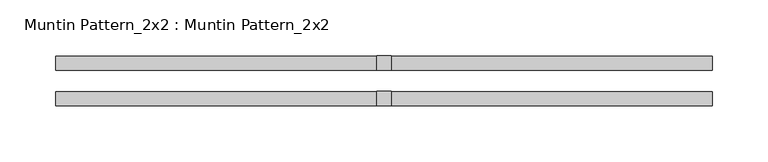
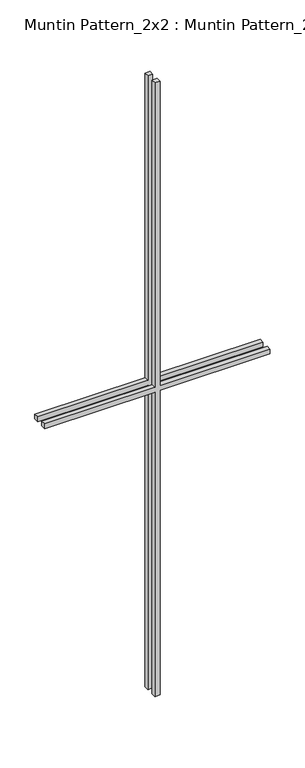
"""IFC4 building model written with IfcOpenShell, lengths in millimetres: proxy geometry, Muntin Pattern_2x2 : Muntin Pattern_2x2."""

from ifc_helpers import new_model, si_unit, frame, origin, place, context, project, spatial, polyline, outline, extrude, source, transform, mapped, element, save


def muntin_pattern_2x2_muntin_pattern_2x2_c2194282(model_context):
    return source(origin(), model_context, "Body", "SweptSolid", [
        extrude(outline(polyline([(850.9, -6.35), (850.9, -293.6875), (838.2, -293.6875), (838.2, -6.35), (0.0, -6.35), (0.0, 6.35), (838.2, 6.35), (838.2, 293.6875), (850.9, 293.6875), (850.9, 6.35), (1689.1, 6.35), (1689.1, -6.35), (850.9, -6.35)])), frame((0.0, -22.225, 0.0), z_axis=(0.0, 1.0, 0.0), x_axis=(0.0, 0.0, 1.0)), (0.0, 0.0, 1.0), 12.7),
        extrude(outline(polyline([(850.9, -6.35), (850.9, -293.6875), (838.2, -293.6875), (838.2, -6.35), (0.0, -6.35), (0.0, 6.35), (838.2, 6.35), (838.2, 293.6875), (850.9, 293.6875), (850.9, 6.35), (1689.1, 6.35), (1689.1, -6.35), (850.9, -6.35)])), frame((0.0, 9.525, 0.0), z_axis=(0.0, 1.0, 0.0), x_axis=(0.0, 0.0, 1.0)), (0.0, 0.0, 1.0), 12.7),
    ])


if __name__ == "__main__":
    model = new_model("IFC4")
    model_context = context("Model", 3, world=origin())
    ifc_project = project(units=[si_unit("LENGTHUNIT", "METRE", prefix="MILLI")], contexts=[model_context])
    site = spatial("IfcSite", under=ifc_project)
    building = spatial("IfcBuilding", under=site)
    placement = place(None, origin())
    muntin_pattern_2x2_muntin_pattern_2x2_shape = muntin_pattern_2x2_muntin_pattern_2x2_c2194282(model_context)
    element("IfcBuildingElementProxy", 1, Name="Muntin Pattern_2x2 : Muntin Pattern_2x2", ObjectType="Muntin Pattern_2x2 : Muntin Pattern_2x2", at=placement, inside=building, context=model_context, shape_type="MappedRepresentation", body=[
        mapped(muntin_pattern_2x2_muntin_pattern_2x2_shape, transform((0.0, 0.0, 0.0), x_axis=(1.0, 0.0, 0.0), y_axis=(0.0, 1.0, 0.0), z_axis=(0.0, 0.0, 1.0))),
    ])
    save(model, "model.ifc")

# Revit data of these elements
# Type "Muntin Pattern_2x2 : Muntin Pattern_2x2"
#   Width [instance default] = 4' - 0"
#   Thickness = 0' - 0 1/2"
#   Height [instance default] = 4' - 0"
#   Distance = 0' - 0 3/4"
#   Interior Material [instance default] = none
#   Exterior Material [instance default] = none
#   Default Elevation = 0
# Element 1 (IfcBuildingElementProxy, "Muntin Pattern_2x2 : Muntin Pattern_2x2")
#   Width = 1' - 11 1/8"
#   Height = 5' - 6 1/2"
#   Interior Material = Wood - Stained
#   Exterior Material = Clad - White
#   Materials on its faces: "Clad - White", "Wood - Stained"
# Materials
#   "Clad - White": class "Wood", colour RGB 242 242 238, transparency 0, Cost = 0
#   "Wood - Stained": class "Wood", colour RGB 224 178 126, transparency 0, Cost = 0
